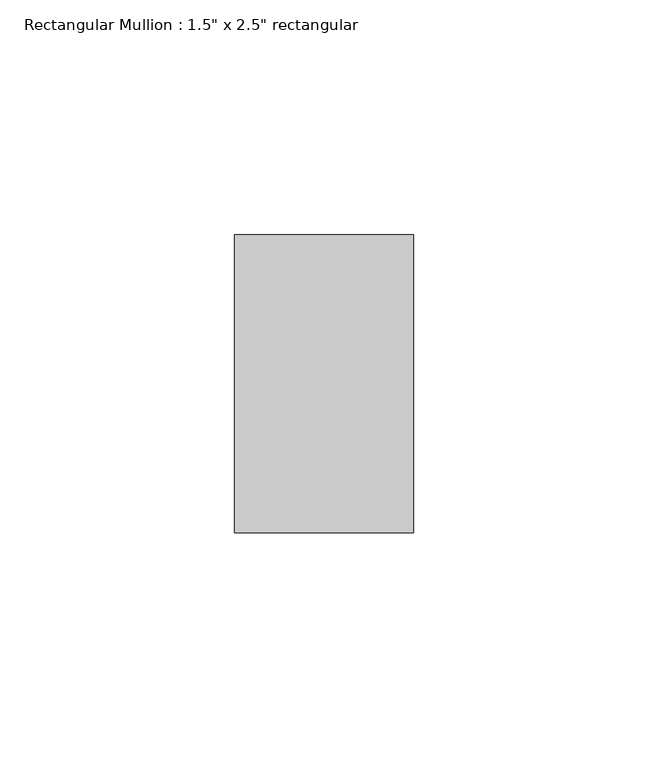
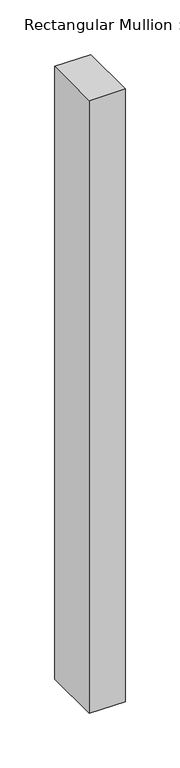
"""IFC4 building model written with IfcOpenShell, lengths in millimetres: member geometry."""

from ifc_helpers import new_model, si_unit, frame, origin, place, context, project, spatial, polyline, outline, extrude, source, transform, mapped, element, save


def member_99569e28(model_context):
    return source(origin(), model_context, "Body", "SweptSolid", [
        extrude(outline(polyline([(0.0, 31.75), (0.0, -31.75), (-38.1, -31.75), (-38.1, 31.75), (0.0, 31.75)])), frame((0.0, 0.0, -685.8), z_axis=(0.0, 0.0, 1.0), x_axis=(1.0, 0.0, 0.0)), (0.0, 0.0, 1.0), 685.8),
    ])


if __name__ == "__main__":
    model = new_model("IFC4")
    model_context = context("Model", 3, world=origin())
    ifc_project = project(units=[si_unit("LENGTHUNIT", "METRE", prefix="MILLI")], contexts=[model_context])
    site = spatial("IfcSite", under=ifc_project)
    building = spatial("IfcBuilding", under=site)
    placement = place(None, origin())
    member_shape = member_99569e28(model_context)
    element("IfcMember", 1, ObjectType="Rectangular Mullion : 1.5\" x 2.5\" rectangular", at=placement, inside=building, context=model_context, shape_type="MappedRepresentation", body=[
        mapped(member_shape, transform((0.0, 0.0, 0.0), x_axis=(1.0, 0.0, 0.0), y_axis=(0.0, 1.0, 0.0), z_axis=(0.0, 0.0, 1.0))),
    ])
    save(model, "model.ifc")

# Revit data of these elements
# Type "Rectangular Mullion : 1.5\" x 2.5\" rectangular"
#   built-in parameter 1007304 = 0.208333 (stored number, unit not read)
#   built-in parameter 1007301 = 0.0625 (stored number, unit not read)
#   built-in parameter 1007300 = 0.0625 (stored number, unit not read)
